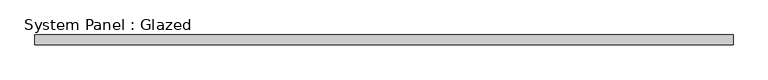
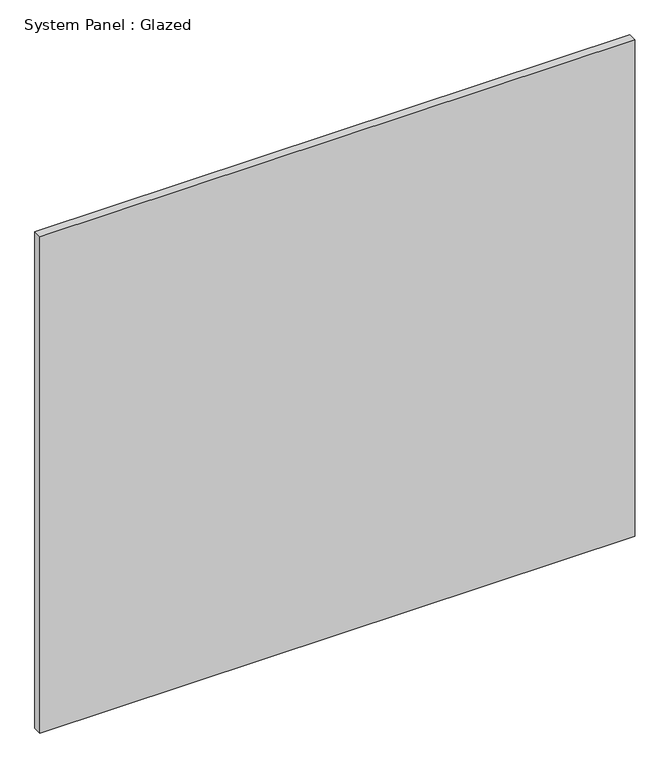
"""IFC4 building model written with IfcOpenShell, lengths in millimetres: plate geometry, System Panel : Glazed."""

from ifc_helpers import new_model, si_unit, origin, origin_with_axes, place, context, project, spatial, polyline, outline, extrude, source, transform, mapped, element, save


def system_panel_glazed_c38f4616(model_context):
    return source(origin(), model_context, "Body", "SweptSolid", [
        extrude(outline(polyline([(912.5143734, 19.05), (-912.5143734, 19.05), (-912.5143734, 44.45), (912.5143734, 44.45), (912.5143734, 19.05)])), origin_with_axes(), (0.0, 0.0, 1.0), 1609.9926716),
    ])


if __name__ == "__main__":
    model = new_model("IFC4")
    model_context = context("Model", 3, world=origin())
    ifc_project = project(units=[si_unit("LENGTHUNIT", "METRE", prefix="MILLI")], contexts=[model_context])
    site = spatial("IfcSite", under=ifc_project)
    building = spatial("IfcBuilding", under=site)
    placement = place(None, origin())
    system_panel_glazed_shape = system_panel_glazed_c38f4616(model_context)
    element("IfcPlate", 1, ObjectType="System Panel : Glazed", at=placement, inside=building, context=model_context, shape_type="MappedRepresentation", body=[
        mapped(system_panel_glazed_shape, transform((0.0, 0.0, 0.0), x_axis=(1.0, 0.0, 0.0), y_axis=(0.0, 1.0, 0.0), z_axis=(0.0, 0.0, 1.0))),
    ])
    save(model, "model.ifc")

# Revit data of these elements
# Type "System Panel : Glazed"
#   Construction Type Id = "GSP4R"
#   Analytic Construction = "1/8 in Pilkington single glazing"
#   Visual Light Transmittance = 0.9
#   Solar Heat Gain Coefficient = 0.86
#   Heat Transfer Coefficient (U) = 1.18115 BTU/(h·ft²·°F)
# Element 1 (IfcPlate, "System Panel : Glazed")
#   Materials on its faces: "Glass"
# Materials
#   "Glass": class "Glass", colour RGB 0 128 192, transparency 0.75, Description = "Soda Lime Glass", Cost = 0
